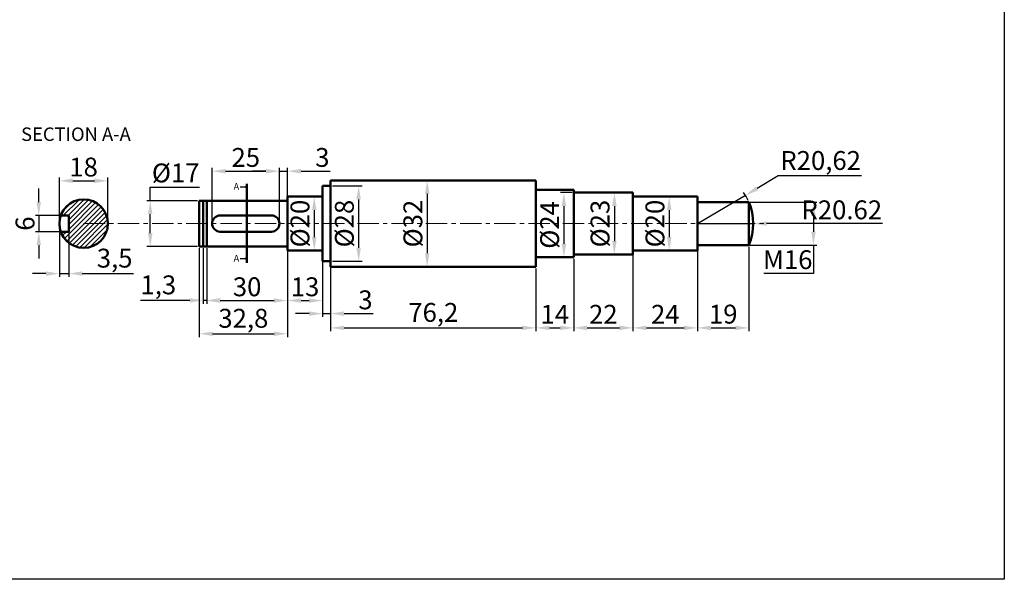
# Model space of a CAD drawing. Units: millimetres. Extents: x -42 to 606, y -195 to 264.
# Tile 2 of 3: x 240 to 606, y -195 to 13. Entities that reach past the tile are written whole.
import ezdxf

# ---------------------------------------------------------------- set-up
doc = ezdxf.new("R2010")
doc.units = ezdxf.units.MM
doc.header["$LTSCALE"] = 0.5
doc.linetypes.add('CENTER', pattern=[50.8, 31.75, -6.35, 6.35, -6.35])
for name, color, linetype, lineweight in [('M-CNTR', 1, 'CENTER', 18), ('M-DIMS', 2, 'Continuous', 25), ('M-HATC', 8, 'Continuous', 18), ('M-OUTL', 7, 'Continuous', 50), ('M-SYMB', 3, 'Continuous', 25), ('M-TEXT', 3, 'Continuous', 25), ('M-TTLB', 7, 'Continuous', 25)]:
    doc.layers.add(name, color=color, linetype=linetype, lineweight=lineweight)
doc.styles.get("Standard").update_dxf_attribs({"font": 'arial.ttf'})
doc.dimstyles.new('ISO-25', dxfattribs={"dimtxt": 7, "dimasz": 5, "dimexe": 1.25, "dimexo": 0.625, "dimtad": 1, "dimtoh": 1, "dimtxsty": 'Standard', "dimcen": 2.5, "dimadec": 0, "dimazin": 0, "dimtfac": 1, "dimtmove": 0, "dimatfit": 3, "dimfxl": 1, "dimarcsym": 0})

# ---------------------------------------------------------------- blocks, each defined once
blk = doc.blocks.new('*D22')
at = {"layer": 'Defpoints', "color": 0, "ltscale": 0.5, "transparency": 16777216}
for p in [(272.82, -46.95), (254.82, -62.83), (272.82, -62.83)]:
    blk.add_point(p, dxfattribs=at)
at = {"layer": 'M-DIMS', "color": 0, "lineweight": -2, "ltscale": 0.5, "transparency": 16777216}
for p, q in [((254.82, -62.2), (254.82, -45.7)), ((259.82, -46.95), (267.82, -46.95)), ((272.82, -62.2), (272.82, -45.7))]:
    blk.add_line(p, q, dxfattribs=at)
at = {"layer": 'M-DIMS', "color": 0, "ltscale": 0.5, "transparency": 16777216}
for points in [[(259.82, -46.11), (259.82, -47.78), (254.82, -46.95)], [(267.82, -46.11), (267.82, -47.78), (272.82, -46.95)]]:
    blk.add_solid(points, dxfattribs=at)
at = {"layer": 'M-DIMS', "color": 0, "ltscale": 0.5, "transparency": 16777216, "insert": (263.82, -42.75), "char_height": 7, "attachment_point": 5}
blk.add_mtext('18', dxfattribs=at)
blk = doc.blocks.new('*D23')
at = {"layer": 'Defpoints', "color": 0, "ltscale": 0.5, "transparency": 16777216}
for p in [(255.34, -59.83), (247.18, -65.83), (255.34, -65.83)]:
    blk.add_point(p, dxfattribs=at)
at = {"layer": 'M-DIMS', "color": 0, "lineweight": -2, "ltscale": 0.5, "transparency": 16777216}
for p, q in [((247.18, -54.83), (247.18, -49.83)), ((254.71, -59.83), (245.93, -59.83)), ((247.18, -59.83), (247.18, -65.83)), ((254.71, -65.83), (245.93, -65.83)), ((247.18, -70.83), (247.18, -75.83))]:
    blk.add_line(p, q, dxfattribs=at)
at = {"layer": 'M-DIMS', "color": 0, "ltscale": 0.5, "transparency": 16777216}
for points in [[(246.34, -54.83), (248.01, -54.83), (247.18, -59.83)], [(246.34, -70.83), (248.01, -70.83), (247.18, -65.83)]]:
    blk.add_solid(points, dxfattribs=at)
at = {"layer": 'M-DIMS', "color": 0, "ltscale": 0.5, "transparency": 16777216, "insert": (242.98, -62.83), "char_height": 7, "attachment_point": 5, "rotation": 90}
blk.add_mtext('6', dxfattribs=at)
blk = doc.blocks.new('*D24')
at = {"layer": 'Defpoints', "color": 0, "ltscale": 0.5, "transparency": 16777216}
for p in [(254.82, -62.83), (258.32, -62.83), (258.32, -81.39)]:
    blk.add_point(p, dxfattribs=at)
at = {"layer": 'M-DIMS', "color": 0, "lineweight": -2, "ltscale": 0.5, "transparency": 16777216}
for p, q in [((254.82, -63.45), (254.82, -82.64)), ((258.32, -63.45), (258.32, -82.64)), ((249.82, -81.39), (244.82, -81.39)), ((254.82, -81.39), (258.32, -81.39)), ((263.32, -81.39), (282.37, -81.39))]:
    blk.add_line(p, q, dxfattribs=at)
at = {"layer": 'M-DIMS', "color": 0, "ltscale": 0.5, "transparency": 16777216}
for points in [[(249.82, -80.56), (249.82, -82.22), (254.82, -81.39)], [(263.32, -80.56), (263.32, -82.22), (258.32, -81.39)]]:
    blk.add_solid(points, dxfattribs=at)
at = {"layer": 'M-DIMS', "color": 0, "ltscale": 0.5, "transparency": 16777216, "insert": (275.34, -76.56), "char_height": 7, "attachment_point": 5}
blk.add_mtext('3,5', dxfattribs=at)
blk = doc.blocks.new('*D25')
at = {"layer": 'Defpoints', "color": 0, "ltscale": 0.5, "transparency": 16777216}
for p in [(306.71, -54.33), (288.55, -71.33), (306.71, -71.33)]:
    blk.add_point(p, dxfattribs=at)
at = {"layer": 'M-DIMS', "color": 0, "lineweight": -2, "ltscale": 0.5, "transparency": 16777216}
for p, q in [((288.55, -54.33), (288.55, -49.33)), ((288.55, -49.33), (306.81, -49.33)), ((306.09, -54.33), (287.3, -54.33)), ((288.55, -66.33), (288.55, -59.33)), ((306.09, -71.33), (287.3, -71.33))]:
    blk.add_line(p, q, dxfattribs=at)
at = {"layer": 'M-DIMS', "color": 0, "ltscale": 0.5, "transparency": 16777216}
for points in [[(287.71, -59.33), (289.38, -59.33), (288.55, -54.33)], [(287.71, -66.33), (289.38, -66.33), (288.55, -71.33)]]:
    blk.add_solid(points, dxfattribs=at)
at = {"layer": 'M-DIMS', "color": 0, "ltscale": 0.5, "transparency": 16777216, "insert": (297.99, -44.93), "char_height": 7, "attachment_point": 5}
blk.add_mtext('%%C17', dxfattribs=at)
blk = doc.blocks.new('*D26')
at = {"layer": 'Defpoints', "color": 0, "ltscale": 0.5, "transparency": 16777216}
for p in [(336.51, -43.38), (311.51, -62.83), (336.51, -62.83)]:
    blk.add_point(p, dxfattribs=at)
at = {"layer": 'M-DIMS', "color": 0, "lineweight": -2, "ltscale": 0.5, "transparency": 16777216}
for p, q in [((311.51, -62.2), (311.51, -42.13)), ((316.51, -43.38), (331.51, -43.38)), ((336.51, -62.2), (336.51, -42.13))]:
    blk.add_line(p, q, dxfattribs=at)
at = {"layer": 'M-DIMS', "color": 0, "ltscale": 0.5, "transparency": 16777216}
for points in [[(316.51, -42.55), (316.51, -44.22), (311.51, -43.38)], [(331.51, -42.55), (331.51, -44.22), (336.51, -43.38)]]:
    blk.add_solid(points, dxfattribs=at)
at = {"layer": 'M-DIMS', "color": 0, "ltscale": 0.5, "transparency": 16777216, "insert": (324.01, -39.18), "char_height": 7, "attachment_point": 5}
blk.add_mtext('25', dxfattribs=at)
blk = doc.blocks.new('*D27')
at = {"layer": 'Defpoints', "color": 0, "ltscale": 0.5, "transparency": 16777216}
for p in [(339.51, -43.38), (336.51, -54.33), (339.51, -54.33)]:
    blk.add_point(p, dxfattribs=at)
at = {"layer": 'M-DIMS', "color": 0, "lineweight": -2, "ltscale": 0.5, "transparency": 16777216}
for p, q in [((331.51, -43.38), (326.51, -43.38)), ((336.51, -53.7), (336.51, -42.13)), ((336.51, -43.38), (339.51, -43.38)), ((339.51, -53.7), (339.51, -42.13)), ((344.51, -43.38), (355.35, -43.38))]:
    blk.add_line(p, q, dxfattribs=at)
at = {"layer": 'M-DIMS', "color": 0, "ltscale": 0.5, "transparency": 16777216}
for points in [[(331.51, -42.55), (331.51, -44.22), (336.51, -43.38)], [(344.51, -42.55), (344.51, -44.22), (339.51, -43.38)]]:
    blk.add_solid(points, dxfattribs=at)
at = {"layer": 'M-DIMS', "color": 0, "ltscale": 0.5, "transparency": 16777216, "insert": (352.43, -39.18), "char_height": 7, "attachment_point": 5}
blk.add_mtext('3', dxfattribs=at)
blk = doc.blocks.new('*D28')
at = {"layer": 'Defpoints', "color": 0, "ltscale": 0.5, "transparency": 16777216}
for p in [(308.21, -71.33), (309.51, -71.33), (309.51, -91.31)]:
    blk.add_point(p, dxfattribs=at)
at = {"layer": 'M-DIMS', "color": 0, "lineweight": -2, "ltscale": 0.5, "transparency": 16777216}
for p, q in [((308.21, -71.95), (308.21, -92.56)), ((309.51, -71.95), (309.51, -92.56)), ((303.21, -91.31), (284.88, -91.31)), ((309.51, -91.31), (308.21, -91.31)), ((314.51, -91.31), (319.51, -91.31))]:
    blk.add_line(p, q, dxfattribs=at)
at = {"layer": 'M-DIMS', "color": 0, "ltscale": 0.5, "transparency": 16777216}
for points in [[(303.21, -90.48), (303.21, -92.14), (308.21, -91.31)], [(314.51, -90.48), (314.51, -92.14), (309.51, -91.31)]]:
    blk.add_solid(points, dxfattribs=at)
at = {"layer": 'M-DIMS', "color": 0, "ltscale": 0.5, "transparency": 16777216, "insert": (291.54, -86.48), "char_height": 7, "attachment_point": 5}
blk.add_mtext('1,3', dxfattribs=at)
blk = doc.blocks.new('*D29')
at = {"layer": 'Defpoints', "color": 0, "ltscale": 0.5, "transparency": 16777216}
for p in [(306.71, -71.33), (339.51, -71.33), (339.51, -103.71)]:
    blk.add_point(p, dxfattribs=at)
at = {"layer": 'M-DIMS', "color": 0, "lineweight": -2, "ltscale": 0.5, "transparency": 16777216}
for p, q in [((306.71, -71.95), (306.71, -104.96)), ((339.51, -71.95), (339.51, -104.96)), ((311.71, -103.71), (334.51, -103.71))]:
    blk.add_line(p, q, dxfattribs=at)
at = {"layer": 'M-DIMS', "color": 0, "ltscale": 0.5, "transparency": 16777216}
for points in [[(311.71, -102.88), (311.71, -104.55), (306.71, -103.71)], [(334.51, -102.88), (334.51, -104.55), (339.51, -103.71)]]:
    blk.add_solid(points, dxfattribs=at)
at = {"layer": 'M-DIMS', "color": 0, "ltscale": 0.5, "transparency": 16777216, "insert": (323.11, -98.88), "char_height": 7, "attachment_point": 5}
blk.add_mtext('32,8', dxfattribs=at)
blk = doc.blocks.new('*D30')
at = {"layer": 'Defpoints', "color": 0, "ltscale": 0.5, "transparency": 16777216}
for p in [(309.51, -71.33), (339.51, -71.33), (339.51, -91.39)]:
    blk.add_point(p, dxfattribs=at)
at = {"layer": 'M-DIMS', "color": 0, "lineweight": -2, "ltscale": 0.5, "transparency": 16777216}
for p, q in [((309.51, -71.95), (309.51, -92.64)), ((339.51, -71.95), (339.51, -92.64)), ((314.51, -91.39), (334.51, -91.39))]:
    blk.add_line(p, q, dxfattribs=at)
at = {"layer": 'M-DIMS', "color": 0, "ltscale": 0.5, "transparency": 16777216}
for points in [[(314.51, -90.56), (314.51, -92.22), (309.51, -91.39)], [(334.51, -90.56), (334.51, -92.22), (339.51, -91.39)]]:
    blk.add_solid(points, dxfattribs=at)
at = {"layer": 'M-DIMS', "color": 0, "ltscale": 0.5, "transparency": 16777216, "insert": (324.51, -87.19), "char_height": 7, "attachment_point": 5}
blk.add_mtext('30', dxfattribs=at)
blk = doc.blocks.new('*D31')
at = {"layer": 'Defpoints', "color": 0, "ltscale": 0.5, "transparency": 16777216}
for p in [(339.51, -72.83), (352.51, -72.83), (352.51, -91.39)]:
    blk.add_point(p, dxfattribs=at)
at = {"layer": 'M-DIMS', "color": 0, "lineweight": -2, "ltscale": 0.5, "transparency": 16777216}
for p, q in [((339.51, -73.45), (339.51, -92.64)), ((352.51, -73.45), (352.51, -92.64)), ((344.51, -91.39), (347.51, -91.39))]:
    blk.add_line(p, q, dxfattribs=at)
at = {"layer": 'M-DIMS', "color": 0, "ltscale": 0.5, "transparency": 16777216}
for points in [[(344.51, -90.56), (344.51, -92.22), (339.51, -91.39)], [(347.51, -90.56), (347.51, -92.22), (352.51, -91.39)]]:
    blk.add_solid(points, dxfattribs=at)
at = {"layer": 'M-DIMS', "color": 0, "ltscale": 0.5, "transparency": 16777216, "insert": (346.01, -87.19), "char_height": 7, "attachment_point": 5}
blk.add_mtext('13', dxfattribs=at)
blk = doc.blocks.new('*D32')
at = {"layer": 'Defpoints', "color": 0, "ltscale": 0.5, "transparency": 16777216}
for p in [(352.51, -52.83), (349.42, -72.83), (352.51, -72.83)]:
    blk.add_point(p, dxfattribs=at)
at = {"layer": 'M-DIMS', "color": 0, "lineweight": -2, "ltscale": 0.5, "transparency": 16777216}
for p, q in [((351.89, -52.83), (348.17, -52.83)), ((349.42, -57.83), (349.42, -67.83)), ((351.89, -72.83), (348.17, -72.83))]:
    blk.add_line(p, q, dxfattribs=at)
at = {"layer": 'M-DIMS', "color": 0, "ltscale": 0.5, "transparency": 16777216}
for points in [[(348.59, -57.83), (350.25, -57.83), (349.42, -52.83)], [(348.59, -67.83), (350.25, -67.83), (349.42, -72.83)]]:
    blk.add_solid(points, dxfattribs=at)
at = {"layer": 'M-DIMS', "color": 0, "ltscale": 0.5, "transparency": 16777216, "insert": (345.02, -62.83), "char_height": 7, "attachment_point": 5, "rotation": 90}
blk.add_mtext('%%C20', dxfattribs=at)
blk = doc.blocks.new('*D33')
at = {"layer": 'Defpoints', "color": 0, "ltscale": 0.5, "transparency": 16777216}
for p in [(355.51, -48.83), (355.51, -76.83), (365.9, -76.83)]:
    blk.add_point(p, dxfattribs=at)
at = {"layer": 'M-DIMS', "color": 0, "lineweight": -2, "ltscale": 0.5, "transparency": 16777216}
for p, q in [((356.14, -48.83), (367.15, -48.83)), ((365.9, -53.83), (365.9, -71.83)), ((356.14, -76.83), (367.15, -76.83))]:
    blk.add_line(p, q, dxfattribs=at)
at = {"layer": 'M-DIMS', "color": 0, "ltscale": 0.5, "transparency": 16777216}
for points in [[(365.06, -53.83), (366.73, -53.83), (365.9, -48.83)], [(365.06, -71.83), (366.73, -71.83), (365.9, -76.83)]]:
    blk.add_solid(points, dxfattribs=at)
at = {"layer": 'M-DIMS', "color": 0, "ltscale": 0.5, "transparency": 16777216, "insert": (361.5, -62.83), "char_height": 7, "attachment_point": 5, "rotation": 90}
blk.add_mtext('%%C28', dxfattribs=at)
blk = doc.blocks.new('*D34')
at = {"layer": 'Defpoints', "color": 0, "ltscale": 0.5, "transparency": 16777216}
for p in [(352.51, -76.83), (355.51, -76.83), (355.51, -96.24)]:
    blk.add_point(p, dxfattribs=at)
at = {"layer": 'M-DIMS', "color": 0, "lineweight": -2, "ltscale": 0.5, "transparency": 16777216}
for p, q in [((352.51, -77.45), (352.51, -97.49)), ((355.51, -77.45), (355.51, -97.49)), ((347.51, -96.24), (342.51, -96.24)), ((352.51, -96.24), (355.51, -96.24)), ((360.51, -96.24), (371.35, -96.24))]:
    blk.add_line(p, q, dxfattribs=at)
at = {"layer": 'M-DIMS', "color": 0, "ltscale": 0.5, "transparency": 16777216}
for points in [[(347.51, -95.41), (347.51, -97.07), (352.51, -96.24)], [(360.51, -95.41), (360.51, -97.07), (355.51, -96.24)]]:
    blk.add_solid(points, dxfattribs=at)
at = {"layer": 'M-DIMS', "color": 0, "ltscale": 0.5, "transparency": 16777216, "insert": (368.43, -92.04), "char_height": 7, "attachment_point": 5}
blk.add_mtext('3', dxfattribs=at)
blk = doc.blocks.new('*D35')
at = {"layer": 'Defpoints', "color": 0, "ltscale": 0.5, "transparency": 16777216}
for p in [(393.61, -46.83), (391.33, -78.83), (393.61, -78.83)]:
    blk.add_point(p, dxfattribs=at)
at = {"layer": 'M-DIMS', "color": 0, "lineweight": -2, "ltscale": 0.5, "transparency": 16777216}
for p, q in [((392.99, -46.83), (390.08, -46.83)), ((391.33, -51.83), (391.33, -73.83)), ((392.99, -78.83), (390.08, -78.83))]:
    blk.add_line(p, q, dxfattribs=at)
at = {"layer": 'M-DIMS', "color": 0, "ltscale": 0.5, "transparency": 16777216}
for points in [[(390.5, -51.83), (392.17, -51.83), (391.33, -46.83)], [(390.5, -73.83), (392.17, -73.83), (391.33, -78.83)]]:
    blk.add_solid(points, dxfattribs=at)
at = {"layer": 'M-DIMS', "color": 0, "ltscale": 0.5, "transparency": 16777216, "insert": (386.94, -62.83), "char_height": 7, "attachment_point": 5, "rotation": 90}
blk.add_mtext('%%C32', dxfattribs=at)
blk = doc.blocks.new('*D36')
at = {"layer": 'Defpoints', "color": 0, "ltscale": 0.5, "transparency": 16777216}
for p in [(355.51, -78.83), (431.71, -78.83), (431.71, -101.54)]:
    blk.add_point(p, dxfattribs=at)
at = {"layer": 'M-DIMS', "color": 0, "lineweight": -2, "ltscale": 0.5, "transparency": 16777216}
for p, q in [((355.51, -79.45), (355.51, -102.79)), ((431.71, -79.45), (431.71, -102.79)), ((360.51, -101.54), (426.71, -101.54))]:
    blk.add_line(p, q, dxfattribs=at)
at = {"layer": 'M-DIMS', "color": 0, "ltscale": 0.5, "transparency": 16777216}
for points in [[(360.51, -100.7), (360.51, -102.37), (355.51, -101.54)], [(426.71, -100.7), (426.71, -102.37), (431.71, -101.54)]]:
    blk.add_solid(points, dxfattribs=at)
at = {"layer": 'M-DIMS', "color": 0, "ltscale": 0.5, "transparency": 16777216, "insert": (393.61, -96.7), "char_height": 7, "attachment_point": 5}
blk.add_mtext('76,2', dxfattribs=at)
blk = doc.blocks.new('*D37')
at = {"layer": 'Defpoints', "color": 0, "ltscale": 0.5, "transparency": 16777216}
for p in [(445.71, -51.33), (442.08, -75.33), (445.71, -75.33)]:
    blk.add_point(p, dxfattribs=at)
at = {"layer": 'M-DIMS', "color": 0, "lineweight": -2, "ltscale": 0.5, "transparency": 16777216}
for p, q in [((445.09, -51.33), (440.83, -51.33)), ((442.08, -56.33), (442.08, -70.33)), ((445.09, -75.33), (440.83, -75.33))]:
    blk.add_line(p, q, dxfattribs=at)
at = {"layer": 'M-DIMS', "color": 0, "ltscale": 0.5, "transparency": 16777216}
for points in [[(441.25, -56.33), (442.91, -56.33), (442.08, -51.33)], [(441.25, -70.33), (442.91, -70.33), (442.08, -75.33)]]:
    blk.add_solid(points, dxfattribs=at)
at = {"layer": 'M-DIMS', "color": 0, "ltscale": 0.5, "transparency": 16777216, "insert": (437.68, -63.33), "char_height": 7, "attachment_point": 5, "rotation": 90}
blk.add_mtext('%%C24', dxfattribs=at)
blk = doc.blocks.new('*D38')
at = {"layer": 'Defpoints', "color": 0, "ltscale": 0.5, "transparency": 16777216}
for p in [(467.71, -52.83), (467.71, -72.83), (481.17, -72.83)]:
    blk.add_point(p, dxfattribs=at)
at = {"layer": 'M-DIMS', "color": 0, "lineweight": -2, "ltscale": 0.5, "transparency": 16777216}
for p, q in [((468.34, -52.83), (482.42, -52.83)), ((481.17, -57.83), (481.17, -67.83)), ((468.34, -72.83), (482.42, -72.83))]:
    blk.add_line(p, q, dxfattribs=at)
at = {"layer": 'M-DIMS', "color": 0, "ltscale": 0.5, "transparency": 16777216}
for points in [[(480.33, -57.83), (482, -57.83), (481.17, -52.83)], [(480.33, -67.83), (482, -67.83), (481.17, -72.83)]]:
    blk.add_solid(points, dxfattribs=at)
at = {"layer": 'M-DIMS', "color": 0, "ltscale": 0.5, "transparency": 16777216, "insert": (476.77, -62.83), "char_height": 7, "width": 10.4793, "attachment_point": 5, "rotation": 90}
blk.add_mtext('%%C20', dxfattribs=at)
blk = doc.blocks.new('*D39')
at = {"layer": 'Defpoints', "color": 0, "ltscale": 0.5, "transparency": 16777216}
for p in [(460.81, -51.33), (460.81, -74.33), (460.81, -74.33)]:
    blk.add_point(p, dxfattribs=at)
at = {"layer": 'M-DIMS', "color": 0, "lineweight": -2, "ltscale": 0.5, "transparency": 16777216}
for p, q in [((461.43, -51.33), (462.06, -51.33)), ((460.81, -56.33), (460.81, -69.33)), ((461.43, -74.33), (462.06, -74.33))]:
    blk.add_line(p, q, dxfattribs=at)
at = {"layer": 'M-DIMS', "color": 0, "ltscale": 0.5, "transparency": 16777216}
for points in [[(459.98, -56.33), (461.64, -56.33), (460.81, -51.33)], [(459.98, -69.33), (461.64, -69.33), (460.81, -74.33)]]:
    blk.add_solid(points, dxfattribs=at)
at = {"layer": 'M-DIMS', "color": 0, "ltscale": 0.5, "transparency": 16777216, "insert": (456.41, -62.83), "char_height": 7, "attachment_point": 5, "rotation": 90}
blk.add_mtext('%%C23', dxfattribs=at)
blk = doc.blocks.new('*D40')
at = {"layer": 'Defpoints', "color": 0, "ltscale": 0.5, "transparency": 16777216}
for p in [(501.21, -54.83), (501.21, -70.83), (534.71, -70.83)]:
    blk.add_point(p, dxfattribs=at)
at = {"layer": 'M-DIMS', "color": 0, "lineweight": -2, "ltscale": 0.5, "transparency": 16777216}
for p, q in [((501.84, -54.83), (535.96, -54.83)), ((534.71, -59.83), (534.71, -65.83)), ((501.84, -70.83), (535.96, -70.83)), ((534.71, -70.83), (534.71, -81.32)), ((534.71, -81.32), (516.24, -81.32))]:
    blk.add_line(p, q, dxfattribs=at)
at = {"layer": 'M-DIMS', "color": 0, "ltscale": 0.5, "transparency": 16777216}
for points in [[(533.88, -59.83), (535.54, -59.83), (534.71, -54.83)], [(533.88, -65.83), (535.54, -65.83), (534.71, -70.83)]]:
    blk.add_solid(points, dxfattribs=at)
at = {"layer": 'M-DIMS', "color": 0, "ltscale": 0.5, "transparency": 16777216, "insert": (525.16, -77.12), "char_height": 7, "attachment_point": 5}
blk.add_mtext('M16', dxfattribs=at)
blk = doc.blocks.new('*D41')
at = {"layer": 'Defpoints', "color": 0, "ltscale": 0.5, "transparency": 16777216}
for p in [(445.71, -75.33), (431.71, -78.83), (445.71, -101.54)]:
    blk.add_point(p, dxfattribs=at)
at = {"layer": 'M-DIMS', "color": 0, "lineweight": -2, "ltscale": 0.5, "transparency": 16777216}
for p, q in [((445.71, -75.95), (445.71, -102.79)), ((431.71, -79.45), (431.71, -102.79)), ((436.71, -101.54), (440.71, -101.54))]:
    blk.add_line(p, q, dxfattribs=at)
at = {"layer": 'M-DIMS', "color": 0, "ltscale": 0.5, "transparency": 16777216}
for points in [[(436.71, -100.7), (436.71, -102.37), (431.71, -101.54)], [(440.71, -100.7), (440.71, -102.37), (445.71, -101.54)]]:
    blk.add_solid(points, dxfattribs=at)
at = {"layer": 'M-DIMS', "color": 0, "ltscale": 0.5, "transparency": 16777216, "insert": (438.71, -97.4), "char_height": 7, "attachment_point": 5}
blk.add_mtext('14', dxfattribs=at)
blk = doc.blocks.new('*D42')
at = {"layer": 'Defpoints', "color": 0, "ltscale": 0.5, "transparency": 16777216}
for p in [(445.71, -75.33), (467.71, -75.33), (467.71, -101.54)]:
    blk.add_point(p, dxfattribs=at)
at = {"layer": 'M-DIMS', "color": 0, "lineweight": -2, "ltscale": 0.5, "transparency": 16777216}
for p, q in [((445.71, -75.95), (445.71, -102.79)), ((467.71, -75.95), (467.71, -102.79)), ((450.71, -101.54), (462.71, -101.54))]:
    blk.add_line(p, q, dxfattribs=at)
at = {"layer": 'M-DIMS', "color": 0, "ltscale": 0.5, "transparency": 16777216}
for points in [[(450.71, -100.7), (450.71, -102.37), (445.71, -101.54)], [(462.71, -100.7), (462.71, -102.37), (467.71, -101.54)]]:
    blk.add_solid(points, dxfattribs=at)
at = {"layer": 'M-DIMS', "color": 0, "ltscale": 0.5, "transparency": 16777216, "insert": (456.71, -97.4), "char_height": 7, "attachment_point": 5}
blk.add_mtext('22', dxfattribs=at)
blk = doc.blocks.new('*D43')
at = {"layer": 'Defpoints', "color": 0, "ltscale": 0.5, "transparency": 16777216}
for p in [(467.71, -72.83), (491.71, -72.83), (491.71, -101.54)]:
    blk.add_point(p, dxfattribs=at)
at = {"layer": 'M-DIMS', "color": 0, "lineweight": -2, "ltscale": 0.5, "transparency": 16777216}
for p, q in [((467.71, -73.45), (467.71, -102.79)), ((491.71, -73.45), (491.71, -102.79)), ((472.71, -101.54), (486.71, -101.54))]:
    blk.add_line(p, q, dxfattribs=at)
at = {"layer": 'M-DIMS', "color": 0, "ltscale": 0.5, "transparency": 16777216}
for points in [[(472.71, -100.7), (472.71, -102.37), (467.71, -101.54)], [(486.71, -100.7), (486.71, -102.37), (491.71, -101.54)]]:
    blk.add_solid(points, dxfattribs=at)
at = {"layer": 'M-DIMS', "color": 0, "ltscale": 0.5, "transparency": 16777216, "insert": (479.71, -97.4), "char_height": 7, "attachment_point": 5}
blk.add_mtext('24', dxfattribs=at)
blk = doc.blocks.new('*D44')
at = {"layer": 'Defpoints', "color": 0, "ltscale": 0.5, "transparency": 16777216}
for p in [(491.71, -70.83), (510.71, -70.83), (510.71, -101.54)]:
    blk.add_point(p, dxfattribs=at)
at = {"layer": 'M-DIMS', "color": 0, "lineweight": -2, "ltscale": 0.5, "transparency": 16777216}
for p, q in [((491.71, -71.45), (491.71, -102.79)), ((510.71, -71.45), (510.71, -102.79)), ((496.71, -101.54), (505.71, -101.54))]:
    blk.add_line(p, q, dxfattribs=at)
at = {"layer": 'M-DIMS', "color": 0, "ltscale": 0.5, "transparency": 16777216}
for points in [[(496.71, -100.7), (496.71, -102.37), (491.71, -101.54)], [(505.71, -100.7), (505.71, -102.37), (510.71, -101.54)]]:
    blk.add_solid(points, dxfattribs=at)
at = {"layer": 'M-DIMS', "color": 0, "ltscale": 0.5, "transparency": 16777216, "insert": (501.21, -97.34), "char_height": 7, "attachment_point": 5}
blk.add_mtext('19', dxfattribs=at)
blk = doc.blocks.new('*D45')
at = {"layer": 'Defpoints', "color": 0, "ltscale": 0.5, "transparency": 16777216}
for p in [(509.46, -52.34), (491.71, -62.83)]:
    blk.add_point(p, dxfattribs=at)
at = {"layer": 'M-DIMS', "color": 0, "lineweight": -2, "ltscale": 0.5, "transparency": 16777216}
for p, q in [((521.62, -45.15), (513.77, -49.8)), ((552.5, -45.15), (521.62, -45.15)), ((491.71, -62.83), (509.46, -52.34))]:
    blk.add_line(p, q, dxfattribs=at)
blk.add_arc((491.71, -62.83), 20.62, 24.5651, 34.0414, dxfattribs=at)
at = {"layer": 'M-DIMS', "color": 0, "ltscale": 0.5, "transparency": 16777216}
blk.add_solid([(513.34, -49.08), (514.19, -50.51), (509.46, -52.34)], dxfattribs=at)
at = {"layer": 'M-DIMS', "color": 0, "ltscale": 0.5, "transparency": 16777216, "insert": (537.37, -40.32), "char_height": 7, "attachment_point": 5}
blk.add_mtext('R20,62', dxfattribs=at)
blk = doc.blocks.new('SECTION-ARROW')
at = {"ltscale": 0.5}
for p, q in [((0, 0.39), (2.47, 0.39)), ((2.47, 0.39), (2.07, 0.78)), ((2.07, 0.78), (2.07, 0)), ((2.47, 0.39), (2.07, 0))]:
    blk.add_line(p, q, dxfattribs=at)
blk = doc.blocks.new('*D79')
at = {"layer": 'Defpoints', "color": 0, "ltscale": 0.5, "transparency": 16777216}
for p in [(491.71, -62.83), (512.33, -62.83)]:
    blk.add_point(p, dxfattribs=at)
at = {"layer": 'M-DIMS', "color": 0, "lineweight": -2, "ltscale": 0.5, "transparency": 16777216}
for p, q in [((491.71, -62.83), (512.33, -62.83)), ((529.47, -62.83), (517.33, -62.83)), ((560.35, -62.83), (529.47, -62.83))]:
    blk.add_line(p, q, dxfattribs=at)
at = {"layer": 'M-DIMS', "color": 0, "ltscale": 0.5, "transparency": 16777216}
blk.add_solid([(517.33, -61.99), (517.33, -63.66), (512.33, -62.83)], dxfattribs=at)
at = {"layer": 'M-DIMS', "color": 0, "ltscale": 0.5, "transparency": 16777216, "insert": (545.22, -58.63), "char_height": 7, "attachment_point": 5}
blk.add_mtext('R20.62', dxfattribs=at)

msp = doc.modelspace()

# ---------------------------------------------------------------- hatches: boundary and pattern name
at = {"layer": 'M-HATC', "ltscale": 0.5}
h = msp.add_hatch(dxfattribs=at)
h.set_pattern_fill('ANSI31', color=256, scale=0.4)
h.paths.add_polyline_path([(255.339, -59.826), (258.324, -59.826), (258.324, -65.826), (255.339, -65.826, 0.843039), (272.824, -62.826, 0.843039)])

# ---------------------------------------------------------------- linework, layer by layer
at = {"layer": 'M-CNTR', "ltscale": 0.5}
msp.add_line((263.824, -62.826), (533.568, -62.826), dxfattribs=at)
at = {"layer": 'M-OUTL', "ltscale": 0.5}
for p, q in [((355.511, -46.826), (355.511, -48.826)), ((355.511, -46.826), (431.711, -46.826)), ((431.711, -46.826), (431.711, -78.826)), ((324.419, -48.067), (324.419, -77.352)), ((355.511, -48.826), (352.511, -48.826)), ((352.511, -48.826), (352.511, -76.826)), ((355.511, -76.826), (355.511, -48.826)), ((431.711, -50.326), (445.711, -50.326)), ((445.711, -50.326), (445.711, -75.326)), ((339.511, -54.326), (306.711, -54.326)), ((306.711, -54.326), (306.711, -71.326)), ((308.211, -71.326), (308.211, -54.326)), ((309.511, -71.326), (309.511, -54.326)), ((352.511, -52.826), (339.511, -52.826)), ((339.511, -52.826), (339.511, -72.826)), ((445.711, -51.326), (467.711, -51.326)), ((467.711, -51.326), (467.711, -74.326)), ((467.711, -52.826), (491.711, -52.826)), ((491.711, -52.826), (491.711, -72.826)), ((491.711, -54.826), (510.711, -54.826)), ((510.711, -54.826), (510.711, -70.826)), ((258.324, -59.826), (255.339, -59.826)), ((258.324, -65.826), (258.324, -59.826)), ((333.511, -59.826), (314.511, -59.826)), ((258.324, -65.826), (255.339, -65.826)), ((314.511, -65.826), (333.511, -65.826)), ((306.711, -71.326), (339.511, -71.326)), ((339.511, -72.826), (352.511, -72.826)), ((491.711, -72.826), (467.711, -72.826)), ((491.711, -70.826), (510.711, -70.826)), ((445.711, -75.326), (431.711, -75.326)), ((467.711, -74.326), (445.711, -74.326)), ((352.511, -76.826), (355.511, -76.826)), ((355.511, -78.826), (355.511, -76.826)), ((431.711, -78.826), (355.511, -78.826))]:
    msp.add_line(p, q, dxfattribs=at)
msp.add_circle((263.824, -62.826), 9, dxfattribs=at)
for centre, radius, start, end in [((491.706, -62.826), 20.62, 337.17158, 22.82842), ((314.511, -62.826), 3, 90, 270), ((333.511, -62.826), 3, 270, 90)]:
    msp.add_arc(centre, radius, start, end, dxfattribs=at)
at = {"layer": 'M-TTLB', "ltscale": 0.5}
msp.add_lwpolyline([(-42.468, 263.673), (605.533, 263.673), (605.533, -194.845), (-42.468, -194.845)], close=True, dxfattribs=at)

# ---------------------------------------------------------------- block references
at = {"layer": 'M-SYMB'}
for p in [(321.953, -49.539), (321.953, -76.208)]:
    msp.add_blockref('SECTION-ARROW', p, dxfattribs=at)

# ---------------------------------------------------------------- texts
at = {"layer": 'M-TEXT', "ltscale": 0.5, "attachment_point": 1}
for s, width, insert, char_height in [('SECTION A-A', 74.73507, (240.615, -27.155), 5), ('A', 3.30931, (319.492, -47.798), 2.5), ('A', 3.30931, (319.492, -74.467), 2.5)]:
    msp.add_mtext_dynamic_manual_height_columns(s, width=width, gutter_width=12.5, heights=[0], dxfattribs=dict(at, insert=insert, char_height=char_height))

# ---------------------------------------------------------------- dimensions: what is measured, and where the dimension line sits
at = {"layer": 'M-DIMS', "ltscale": 0.5}
for base, p1, p2, picture, middle in [((336.511, -43.383), (311.511, -62.826), (336.511, -62.826), '*D26', (324.011, -39.184)), ((339.511, -43.383), (336.511, -54.326), (339.511, -54.326), '*D27', (352.428, -39.181)), ((272.824, -46.946), (254.824, -62.826), (272.824, -62.826), '*D22', (263.824, -42.747)), ((258.324, -81.39), (254.824, -62.826), (258.324, -62.826), '*D24', (275.345, -76.558)), ((339.511, -103.713), (306.711, -71.326), (339.511, -71.326), '*D29', (323.111, -98.881)), ((339.511, -91.392), (309.511, -71.326), (339.511, -71.326), '*D30', (324.511, -87.19)), ((352.511, -91.392), (339.511, -72.826), (352.511, -72.826), '*D31', (346.011, -87.19)), ((491.711, -101.536), (467.711, -72.826), (491.711, -72.826), '*D43', (479.711, -97.397)), ((510.711, -101.536), (491.711, -70.826), (510.711, -70.826), '*D44', (501.211, -97.337)), ((445.711, -101.536), (431.711, -78.826), (445.711, -75.326), '*D41', (438.711, -97.397)), ((467.711, -101.536), (445.711, -75.326), (467.711, -75.326), '*D42', (456.711, -97.397)), ((355.511, -96.241), (352.511, -76.826), (355.511, -76.826), '*D34', (368.428, -92.039)), ((431.711, -101.536), (355.511, -78.826), (431.711, -78.826), '*D36', (393.611, -96.704))]:
    dim = msp.add_linear_dim(base=base, p1=p1, p2=p2, dimstyle='ISO-25', override={"dimclrd": 0, "dimclre": 0, "dimclrt": 0}, dxfattribs=at)
    dim.commit()
    dim.dimension.update_dxf_attribs({"geometry": picture, "text_midpoint": middle})
dim = msp.add_radius_dim(center=(491.706, -62.826), mpoint=(509.461, -52.339), dimstyle='ISO-25', override={"dimclrd": 0, "dimclre": 0, "dimclrt": 0}, dxfattribs=at)
dim.commit()
dim.dimension.update_dxf_attribs({"geometry": '*D45', "text_midpoint": (537.374, -45.155), "dimtype": 164})
for base, p1, p2, text, picture, middle in [((288.547, -71.326), (306.711, -54.326), (306.711, -71.326), '%%C<>', '*D25', (297.993, -49.326)), ((534.711, -70.826), (501.211, -54.826), (501.211, -70.826), 'M<>', '*D40', (525.161, -81.32))]:
    dim = msp.add_linear_dim(base=base, p1=p1, p2=p2, angle=90, text=text, dimstyle='ISO-25', override={"dimclrd": 0, "dimclre": 0, "dimclrt": 0}, dxfattribs=at)
    dim.commit()
    dim.dimension.update_dxf_attribs({"geometry": picture, "text_midpoint": middle, "dimtype": 160})
for base, p1, p2, picture, middle in [((391.333, -78.826), (393.611, -46.826), (393.611, -78.826), '*D35', (386.938, -62.826)), ((365.895, -76.826), (355.511, -48.826), (355.511, -76.826), '*D33', (361.501, -62.826)), ((349.42, -72.826), (352.511, -52.826), (352.511, -72.826), '*D32', (345.025, -62.826)), ((442.08, -75.326), (445.711, -51.326), (445.711, -75.326), '*D37', (437.685, -63.326)), ((460.808, -74.326), (460.808, -51.326), (460.808, -74.326), '*D39', (456.414, -62.826)), ((481.166, -72.826), (467.711, -52.826), (467.711, -72.826), '*D38', (476.771, -62.826))]:
    dim = msp.add_linear_dim(base=base, p1=p1, p2=p2, angle=90, text='%%C<>', dimstyle='ISO-25', override={"dimclrd": 0, "dimclre": 0, "dimclrt": 0}, dxfattribs=at)
    dim.commit()
    dim.dimension.update_dxf_attribs({"geometry": picture, "text_midpoint": middle})
dim = msp.add_linear_dim(base=(247.175, -65.826), p1=(255.339, -59.826), p2=(255.339, -65.826), angle=90, dimstyle='ISO-25', override={"dimclrd": 0, "dimclre": 0, "dimclrt": 0}, dxfattribs=at)
dim.commit()
dim.dimension.update_dxf_attribs({"geometry": '*D23', "text_midpoint": (242.976, -62.826)})
dim = msp.add_radius_dim(center=(491.706, -62.826), mpoint=(512.326, -62.826), dimstyle='ISO-25', override={"dimdec": 2, "dimlfac": 1, "dimrnd": 0, "dimzin": 0, "dimdsep": 46, "dimlunit": 2}, dxfattribs=at)
dim.commit()
dim.dimension.update_dxf_attribs({"geometry": '*D79', "text_midpoint": (545.224, -58.627)})
dim = msp.add_linear_dim(base=(309.511, -91.31), p1=(308.211, -71.326), p2=(309.511, -71.326), dimstyle='ISO-25', override={"dimclrd": 0, "dimclre": 0, "dimclrt": 0}, dxfattribs=at)
dim.commit()
dim.dimension.update_dxf_attribs({"geometry": '*D28', "text_midpoint": (291.543, -91.31), "dimtype": 160})

doc.saveas('drawing.dxf')
